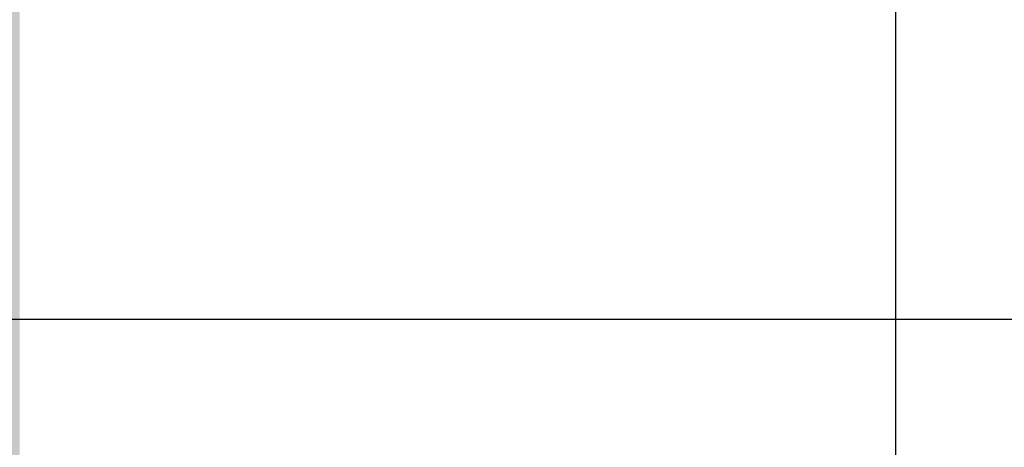
# Model space of a CAD drawing. Units: inches. Extents: x 2696 to 3240, y 1564 to 2310.
# Tile 41 of 76: x 2755 to 2786, y 2071 to 2084. Entities that reach past the tile are written whole.
import ezdxf

# ---------------------------------------------------------------- set-up
doc = ezdxf.new("R2010")
doc.units = ezdxf.units.IN
doc.layers.add('A-ANNO-DIMS', color=3, linetype='Continuous', lineweight=18)
doc.layers.add('A-WALL-PATT', color=9, linetype='Continuous', lineweight=13)
doc.styles.add('TIMES NEW', font='times.ttf')
doc.dimstyles.new('Siddhuu', dxfattribs={"dimtxt": 6, "dimasz": 2.5, "dimexe": 1.25, "dimexo": 0.625, "dimtad": 1, "dimdec": 1, "dimlunit": 4, "dimtxsty": 'TIMES NEW', "dimcen": 2.5, "dimclrd": 256, "dimclre": 1, "dimclrt": 7, "dimadec": 0, "dimazin": 0, "dimtfac": 1, "dimtdec": 1, "dimtmove": 0, "dimatfit": 3, "dimfxl": 1, "dimtolj": 1, "dimlwd": -1, "dimarcsym": 0})

# ---------------------------------------------------------------- blocks, each defined once
blk = doc.blocks.new('*D40')
at = {"layer": 'A-ANNO-DIMS', "color": 1, "lineweight": -2, "transparency": 16777216}
for p, q in [((2777.266, 2091.826), (2777.266, 2093.576)), ((2784.764, 2091.826), (2784.764, 2093.576))]:
    blk.add_line(p, q, dxfattribs=at)
at = {"layer": 'A-ANNO-DIMS', "transparency": 16777216}
for p, q in [((2779.766, 2092.326), (2782.264, 2092.326)), ((2784.764, 2092.326), (2902.458, 2092.326))]:
    blk.add_line(p, q, dxfattribs=at)
for points in [[(2779.766, 2092.742), (2779.766, 2091.909), (2777.266, 2092.326)], [(2782.264, 2092.742), (2782.264, 2091.909), (2784.764, 2092.326)]]:
    blk.add_solid(points, dxfattribs=at)
at = {"layer": 'Defpoints', "color": 0, "transparency": 16777216}
for p in [(2784.764, 2092.326), (2777.266, 2091.201), (2784.764, 2091.201)]:
    blk.add_point(p, dxfattribs=at)
at = {"layer": 'A-ANNO-DIMS', "color": 7, "transparency": 16777216, "insert": (2844.861, 2096.094), "char_height": 6, "attachment_point": 5, "style": 'TIMES NEW'}
blk.add_mtext('\\A1;BATH FITTING 0\'-7 1/2" TYP.', dxfattribs=at)
blk = doc.blocks.new('*D62')
at = {"layer": 'A-ANNO-DIMS', "color": 1, "lineweight": -2, "transparency": 16777216}
for p, q in [((2965.084, 2140.701), (2709.361, 2140.701)), ((2965.084, 2063.591), (2709.361, 2063.591))]:
    blk.add_line(p, q, dxfattribs=at)
at = {"layer": 'A-ANNO-DIMS', "transparency": 16777216}
blk.add_line((2710.611, 2066.091), (2710.611, 2138.201), dxfattribs=at)
for points in [[(2710.195, 2138.201), (2711.028, 2138.201), (2710.611, 2140.701)], [(2710.195, 2066.091), (2711.028, 2066.091), (2710.611, 2063.591)]]:
    blk.add_solid(points, dxfattribs=at)
at = {"layer": 'Defpoints', "color": 0, "transparency": 16777216}
for p in [(2710.611, 2140.701), (2965.709, 2140.701), (2965.709, 2063.591)]:
    blk.add_point(p, dxfattribs=at)
at = {"layer": 'A-ANNO-DIMS', "color": 7, "transparency": 16777216, "insert": (2706.934, 2102.146), "char_height": 6, "attachment_point": 5, "rotation": 90, "style": 'TIMES NEW'}
blk.add_mtext('\\A1;6\'-5"', dxfattribs=at)
blk = doc.blocks.new('*D64')
at = {"layer": 'A-ANNO-DIMS', "color": 1, "lineweight": -2, "transparency": 16777216}
for p, q in [((3073.084, 2206.701), (2709.361, 2206.701)), ((3068.584, 1989.201), (2709.361, 1989.201))]:
    blk.add_line(p, q, dxfattribs=at)
at = {"layer": 'A-ANNO-DIMS', "transparency": 16777216}
blk.add_line((2710.611, 1991.701), (2710.611, 2204.201), dxfattribs=at)
for points in [[(2710.195, 2204.201), (2711.028, 2204.201), (2710.611, 2206.701)], [(2710.195, 1991.701), (2711.028, 1991.701), (2710.611, 1989.201)]]:
    blk.add_solid(points, dxfattribs=at)
at = {"layer": 'Defpoints', "color": 0, "transparency": 16777216}
for p in [(2710.611, 2206.701), (3073.709, 2206.701), (3069.209, 1989.201)]:
    blk.add_point(p, dxfattribs=at)
at = {"layer": 'A-ANNO-DIMS', "color": 7, "transparency": 16777216, "insert": (2706.85, 2097.951), "char_height": 6, "attachment_point": 5, "rotation": 90, "style": 'TIMES NEW'}
blk.add_mtext('\\A1;18\'-1 1/2"', dxfattribs=at)
blk = doc.blocks.new('*D66')
at = {"layer": 'A-ANNO-DIMS', "color": 1, "lineweight": -2, "transparency": 16777216}
for p, q in [((3077.584, 2122.701), (2709.361, 2122.701)), ((3077.584, 2074.701), (2709.361, 2074.701))]:
    blk.add_line(p, q, dxfattribs=at)
at = {"layer": 'A-ANNO-DIMS', "transparency": 16777216}
blk.add_line((2710.611, 2077.201), (2710.611, 2120.201), dxfattribs=at)
for points in [[(2710.195, 2120.201), (2711.028, 2120.201), (2710.611, 2122.701)], [(2710.195, 2077.201), (2711.028, 2077.201), (2710.611, 2074.701)]]:
    blk.add_solid(points, dxfattribs=at)
at = {"layer": 'Defpoints', "color": 0, "transparency": 16777216}
for p in [(2710.611, 2122.701), (3078.209, 2122.701), (3078.209, 2074.701)]:
    blk.add_point(p, dxfattribs=at)
at = {"layer": 'A-ANNO-DIMS', "color": 7, "transparency": 16777216, "insert": (2706.934, 2098.701), "char_height": 6, "attachment_point": 5, "rotation": 90, "style": 'TIMES NEW'}
blk.add_mtext('\\A1;4\'-0"', dxfattribs=at)
blk = doc.blocks.new('*D68')
at = {"layer": 'A-ANNO-DIMS', "color": 1, "lineweight": -2, "transparency": 16777216}
for p, q in [((2745.611, 2261.576), (2745.611, 1568.951)), ((2782.834, 2261.576), (2782.834, 1568.951))]:
    blk.add_line(p, q, dxfattribs=at)
at = {"layer": 'A-ANNO-DIMS', "transparency": 16777216}
blk.add_line((2748.111, 1570.201), (2780.334, 1570.201), dxfattribs=at)
for points in [[(2748.111, 1570.618), (2748.111, 1569.784), (2745.611, 1570.201)], [(2780.334, 1570.618), (2780.334, 1569.784), (2782.834, 1570.201)]]:
    blk.add_solid(points, dxfattribs=at)
at = {"layer": 'Defpoints', "color": 0, "transparency": 16777216}
for p in [(2745.611, 2262.201), (2782.834, 2262.201), (2782.834, 1570.201)]:
    blk.add_point(p, dxfattribs=at)
at = {"layer": 'A-ANNO-DIMS', "color": 7, "transparency": 16777216, "insert": (2764.223, 1573.878), "char_height": 6, "attachment_point": 5, "style": 'TIMES NEW'}
blk.add_mtext('\\A1;3\'-1"', dxfattribs=at)

msp = doc.modelspace()

# ---------------------------------------------------------------- hatches: boundary and pattern name
at = {"layer": 'A-WALL-PATT', "transparency": 33554556}
h = msp.add_hatch(color=256, dxfattribs=at)
h.dxf.hatch_style = 1
h.paths.add_polyline_path([(2879.111, 2253.201), (2905.91, 2253.201), (2905.91, 2262.201), (2841.889, 2262.201), (2841.889, 2253.201), (2870.111, 2253.201), (2870.111, 2176.601), (2965.709, 2176.601), (2965.709, 2206.701), (2973.583, 2206.701), (2973.583, 2215.701), (2965.709, 2215.701), (2965.709, 2262.201), (2929.91, 2262.201), (2929.91, 2253.201), (2956.709, 2253.201), (2956.709, 2185.601), (2879.111, 2185.601)])
h.paths.add_polyline_path([(2782.834, 2262.201), (2745.611, 2262.201), (2745.611, 2228.729), (2754.611, 2228.729), (2754.611, 2253.201), (2782.834, 2253.201)])
h.paths.add_polyline_path([(2754.611, 2136.201), (2965.709, 2136.201), (2965.709, 2145.201), (2879.111, 2145.201), (2879.111, 2147.074), (2877.34, 2147.074), (2870.111, 2147.074), (2870.111, 2145.201), (2754.611, 2145.201), (2754.611, 2169.674), (2745.611, 2169.674), (2745.611, 2000.201), (2754.611, 2000.201), (2754.611, 2019.201), (2849.083, 2019.201), (2849.083, 2023.701), (2841.209, 2023.701), (2841.209, 2051.827), (2836.709, 2051.827), (2836.709, 2023.701), (2754.611, 2023.701), (2754.611, 2091.201), (2836.709, 2091.201), (2836.709, 2087.827), (2841.209, 2087.827), (2841.209, 2095.701), (2754.611, 2095.701)])
h.paths.add_polyline_path([(2965.709, 2136.201), (2956.709, 2136.201), (2956.709, 2023.701), (2885.083, 2023.701), (2885.083, 2019.201), (2956.709, 2019.201), (2956.709, 1950.575), (2965.709, 1950.575), (2965.709, 1980.201), (2973.583, 1980.201), (2973.583, 1989.201), (2965.709, 1989.201)])
h.paths.add_polyline_path([(2754.611, 1906.701), (2880.209, 1906.701), (2884.709, 1906.701), (2956.709, 1906.701), (2956.709, 1792.701), (2944.709, 1792.701), (2944.709, 1783.701), (2956.709, 1783.701), (2956.709, 1740.201), (2884.709, 1740.201), (2884.709, 1783.701), (2896.709, 1783.701), (2896.709, 1792.701), (2884.709, 1792.701), (2884.709, 1846.701), (2880.209, 1846.701), (2880.209, 1740.201), (2754.611, 1740.201), (2754.611, 1777.201), (2745.611, 1777.201), (2745.611, 1692.701), (2754.611, 1692.701), (2754.611, 1731.201), (2956.709, 1731.201), (2956.709, 1723.327), (2965.709, 1723.327), (2965.709, 1884.201), (2973.583, 1884.201), (2973.583, 1893.201), (2965.709, 1893.201), (2965.709, 1914.575), (2956.709, 1914.575), (2956.709, 1911.201), (2754.611, 1911.201), (2754.611, 1930.201), (2745.611, 1930.201), (2745.611, 1817.201), (2754.611, 1817.201), (2754.611, 1854.201), (2826.611, 1854.201), (2826.611, 1868.827), (2822.111, 1868.827), (2822.111, 1858.701), (2754.611, 1858.701)])
h.paths.add_polyline_path([(2965.709, 1656.201), (3008.237, 1656.201), (3008.237, 1665.201), (2965.709, 1665.201), (2965.709, 1693.327), (2956.709, 1693.327), (2956.709, 1686.201), (2934.583, 1686.201), (2934.583, 1681.701), (2956.709, 1681.701), (2956.709, 1614.201), (2896.709, 1614.201), (2896.709, 1681.701), (2904.583, 1681.701), (2904.583, 1686.201), (2892.209, 1686.201), (2892.209, 1614.201), (2858.41, 1614.201), (2858.41, 1605.201), (2965.709, 1605.201)])
h.paths.add_polyline_path([(2788.41, 1614.201), (2754.611, 1614.201), (2754.611, 1652.701), (2745.611, 1652.701), (2745.611, 1605.201), (2788.41, 1605.201)])
h.paths.add_polyline_path([(3199.611, 1633.048), (3190.611, 1633.048), (3190.611, 1614.201), (3082.611, 1614.201), (3082.611, 1665.201), (3070.237, 1665.201), (3070.237, 1656.201), (3078.111, 1656.201), (3078.111, 1605.201), (3199.611, 1605.201)])
h.paths.add_polyline_path([(3199.611, 1702.048), (3190.611, 1702.048), (3190.611, 1699.701), (3106.611, 1699.701), (3106.611, 1747.701), (3190.611, 1747.701), (3190.611, 1752.201), (3082.611, 1752.201), (3082.611, 1760.075), (3078.111, 1760.075), (3078.111, 1747.701), (3102.111, 1747.701), (3102.111, 1699.701), (3078.111, 1699.701), (3078.111, 1695.201), (3190.611, 1695.201), (3190.611, 1676.355), (3199.611, 1676.355)])
h.paths.add_polyline_path([(3199.611, 1783.201), (3190.611, 1783.201), (3190.611, 1745.355), (3199.611, 1745.355)])
h.paths.add_polyline_path([(3082.611, 1884.201), (3190.611, 1884.201), (3190.611, 1853.201), (3199.611, 1853.201), (3199.611, 1901.701), (3190.611, 1901.701), (3190.611, 1893.201), (3005.583, 1893.201), (3005.583, 1891.281), (3005.583, 1884.201), (3078.111, 1884.201), (3078.111, 1792.075), (3082.611, 1792.075)])
h.paths.add_polyline_path([(3199.611, 1994.701), (3190.611, 1994.701), (3190.611, 1989.201), (3073.709, 1989.201), (3073.709, 2034.201), (3069.209, 2034.201), (3069.209, 1989.201), (3005.583, 1989.201), (3005.583, 1980.201), (3190.611, 1980.201), (3190.611, 1971.701), (3199.611, 1971.701)])
h.paths.add_polyline_path([(3199.611, 2155.201), (3190.611, 2155.201), (3190.611, 2064.701), (3199.611, 2064.701)])
h.paths.add_polyline_path([(3190.611, 2074.701), (3106.611, 2074.701), (3106.611, 2122.701), (3190.611, 2122.701), (3190.611, 2127.201), (3082.709, 2127.201), (3082.709, 2135.075), (3073.709, 2135.075), (3073.709, 2122.701), (3102.111, 2122.701), (3102.111, 2074.701), (3069.209, 2074.701), (3069.209, 2070.201), (3190.611, 2070.201)])
h.paths.add_polyline_path([(3082.709, 2253.201), (3190.611, 2253.201), (3190.611, 2225.201), (3199.611, 2225.201), (3199.611, 2262.201), (3073.709, 2262.201), (3073.709, 2215.701), (3035.583, 2215.701), (3035.583, 2206.701), (3073.709, 2206.701), (3073.709, 2171.075), (3082.709, 2171.075)])

# ---------------------------------------------------------------- dimensions: what is measured, and where the dimension line sits
at = {"layer": 'A-ANNO-DIMS'}
dim = msp.add_linear_dim(base=(2782.834, 1570.201), p1=(2745.611, 2262.201), p2=(2782.834, 2262.201), dimstyle='Siddhuu', override={"dimdec": 1, "dimlfac": 1, "dimrnd": 0, "dimzin": 1, "dimdsep": 46, "dimlunit": 4, "dimfrac": 2}, dxfattribs=at)
dim.commit()
dim.dimension.update_dxf_attribs({"geometry": '*D68', "text_midpoint": (2764.223, 1573.878)})
for base, p1, p2, picture, middle in [((2710.611, 2206.701), (3069.209, 1989.201), (3073.709, 2206.701), '*D64', (2706.85, 2097.951)), ((2710.611, 2140.701), (2965.709, 2063.591), (2965.709, 2140.701), '*D62', (2706.934, 2102.146)), ((2710.611, 2122.701), (3078.209, 2074.701), (3078.209, 2122.701), '*D66', (2706.934, 2098.701))]:
    dim = msp.add_linear_dim(base=base, p1=p1, p2=p2, angle=90, dimstyle='Siddhuu', override={"dimdec": 1, "dimlfac": 1, "dimrnd": 0, "dimzin": 1, "dimdsep": 46, "dimlunit": 4, "dimfrac": 2}, dxfattribs=at)
    dim.commit()
    dim.dimension.update_dxf_attribs({"geometry": picture, "text_midpoint": middle})
dim = msp.add_linear_dim(base=(2784.764, 2092.326), p1=(2777.266, 2091.201), p2=(2784.764, 2091.201), text='BATH FITTING <> TYP.', dimstyle='Siddhuu', override={"dimdec": 1, "dimlfac": 1, "dimrnd": 0, "dimzin": 1, "dimdsep": 46, "dimlunit": 4, "dimfrac": 2}, dxfattribs=at)
dim.commit()
dim.dimension.update_dxf_attribs({"geometry": '*D40', "text_midpoint": (2844.861, 2096.094)})

doc.saveas('drawing.dxf')
